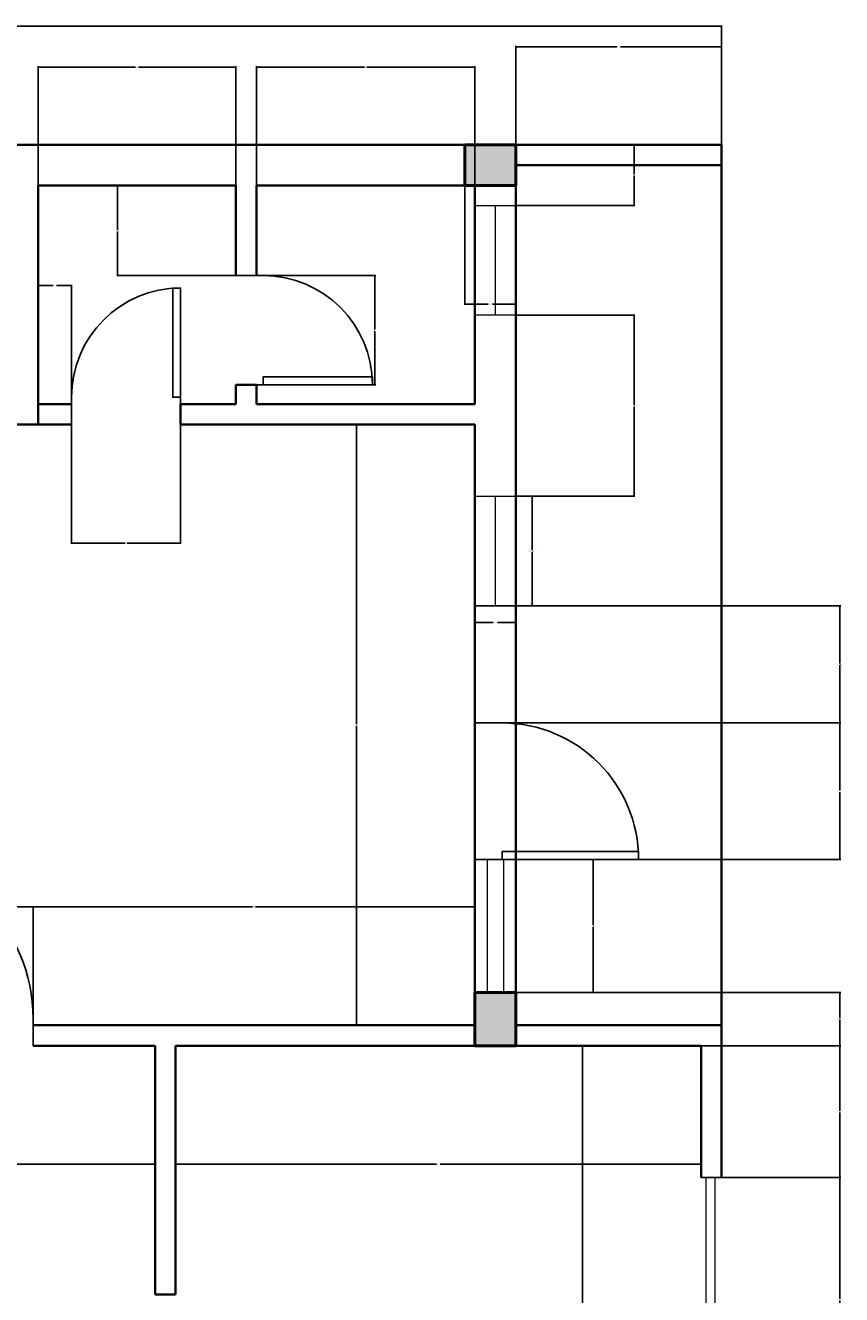
# Model space of a CAD drawing. Units: inches. Extents: x 229 to 651, y 108 to 681.
# Tile 4 of 4: x 472 to 651, y 402 to 681. Entities that reach past the tile are written whole.
import ezdxf

# ---------------------------------------------------------------- set-up
doc = ezdxf.new("R2010")
doc.units = ezdxf.units.IN
doc.header["$MEASUREMENT"] = 0
for name, color, linetype, lineweight in [('A-ANNO-DIMS', 2, 'Continuous', 18), ('A-COLS', 7, 'Continuous', 50), ('A-COLS-PATT', 5, 'Continuous', 13), ('A-DOOR', 3, 'Continuous', 25), ('A-GLAZ', 4, 'Continuous', 18), ('A-WALL', 7, 'Continuous', 35)]:
    doc.layers.add(name, color=color, linetype=linetype, lineweight=lineweight)
doc.styles.get("Standard").update_dxf_attribs({"font": 'arial.ttf'})
doc.dimstyles.get("Standard").update_dxf_attribs({"dimtxt": 0.18, "dimasz": 0.18, "dimexe": 0.18, "dimexo": 0.0625, "dimgap": 0.09, "dimtad": 0, "dimtih": 1, "dimtoh": 1, "dimdec": 4, "dimzin": 0, "dimdsep": 46, "dimtxsty": 'Standard', "dimcen": 0.09, "dimadec": 0, "dimazin": 0, "dimtfac": 1, "dimtdec": 4, "dimtofl": 0, "dimtmove": 0, "dimatfit": 3, "dimfxl": 1, "dimtolj": 1, "dimtzin": 0, "dimarcsym": 0})

# ---------------------------------------------------------------- blocks, each defined once
blk = doc.blocks.new('*U4')
for p, q in [((0, 0), (0, -6)), ((36, 0), (36, -6))]:
    blk.add_line(p, q)
blk.add_lwpolyline([(0, 0), (0, 36), (1.75, 36), (1.75, 0)], close=True)
blk.add_arc((0, 0), 36, 0, 90)
blk = doc.blocks.new('*U5')
for p, q in [((-24, 0), (-24, -6)), ((0, 0), (0, -6))]:
    blk.add_line(p, q)
blk.add_lwpolyline([(0, 0), (0, 24), (-1.75, 24), (-1.75, 0)], close=True)
blk.add_arc((0, 0), 24, 90, 180)
blk = doc.blocks.new('*U6')
for p, q in [((-30, 0), (-30, -6)), ((0, 0), (0, -6))]:
    blk.add_line(p, q)
blk.add_lwpolyline([(0, 0), (0, 30), (-1.75, 30), (-1.75, 0)], close=True)
blk.add_arc((0, 0), 30, 90, 180)
blk = doc.blocks.new('WIN-24IN-SINGLE')
for p, q in [((0, 24.08), (9, 24.08)), ((0, 0), (0, 24.08)), ((0, 24.08), (4.5, 24.08)), ((4.5, 24.08), (4.5, 0)), ((9, 24.08), (9, 0)), ((9, 0), (0, 0))]:
    blk.add_line(p, q)
blk = doc.blocks.new('*D11')
at = {"layer": 'A-ANNO-DIMS', "color": 0, "lineweight": -2, "transparency": 16777216}
for p, q in [((579.81, 577.83), (583.54, 577.83)), ((583.36, 577.65), (583.36, 565.97)), ((583.36, 553.93), (583.36, 565.6)), ((579.81, 553.75), (583.54, 553.75))]:
    blk.add_line(p, q, dxfattribs=at)
at = {"layer": 'A-ANNO-DIMS', "color": 0, "transparency": 16777216}
for points in [[(583.33, 577.65), (583.39, 577.65), (583.36, 577.83)], [(583.33, 553.93), (583.39, 553.93), (583.36, 553.75)]]:
    blk.add_solid(points, dxfattribs=at)
at = {"layer": 'Defpoints', "color": 0, "transparency": 16777216}
for p in [(579.74, 577.83), (583.36, 577.83), (579.74, 553.75)]:
    blk.add_point(p, dxfattribs=at)
at = {"layer": 'A-ANNO-DIMS', "color": 0, "transparency": 16777216, "insert": (583.36, 565.79), "char_height": 0.18, "attachment_point": 5}
blk.add_mtext('\\A1;WINDOW 24 TYP.', dxfattribs=at)
blk = doc.blocks.new('*D12')
at = {"layer": 'A-ANNO-DIMS', "color": 0, "lineweight": -2, "transparency": 16777216}
for p, q in [((570.74, 553.68), (570.74, 549.95)), ((579.74, 553.68), (579.74, 549.95)), ((570.92, 550.13), (574.79, 550.13)), ((579.56, 550.13), (575.7, 550.13))]:
    blk.add_line(p, q, dxfattribs=at)
at = {"layer": 'A-ANNO-DIMS', "color": 0, "transparency": 16777216}
for points in [[(570.92, 550.16), (570.92, 550.1), (570.74, 550.13)], [(579.56, 550.16), (579.56, 550.1), (579.74, 550.13)]]:
    blk.add_solid(points, dxfattribs=at)
at = {"layer": 'Defpoints', "color": 0, "transparency": 16777216}
for p in [(570.74, 553.75), (579.74, 553.75), (579.74, 550.13)]:
    blk.add_point(p, dxfattribs=at)
at = {"layer": 'A-ANNO-DIMS', "color": 0, "transparency": 16777216, "insert": (575.24, 550.13), "char_height": 0.18, "attachment_point": 5}
blk.add_mtext('\\A1;9 TYP.', dxfattribs=at)
blk = doc.blocks.new('*D13')
at = {"layer": 'A-ANNO-DIMS', "color": 0, "lineweight": -2, "transparency": 16777216}
for p, q in [((255.74, 655.15), (255.74, 681.3)), ((255.92, 681.12), (439.96, 681.12)), ((624.79, 681.12), (440.75, 681.12)), ((624.97, 655.15), (624.97, 681.3))]:
    blk.add_line(p, q, dxfattribs=at)
at = {"layer": 'A-ANNO-DIMS', "color": 0, "transparency": 16777216}
for points in [[(255.92, 681.15), (255.92, 681.09), (255.74, 681.12)], [(624.79, 681.15), (624.79, 681.09), (624.97, 681.12)]]:
    blk.add_solid(points, dxfattribs=at)
at = {"layer": 'Defpoints', "color": 0, "transparency": 16777216}
for p in [(624.97, 681.12), (255.74, 655.09), (624.97, 655.09)]:
    blk.add_point(p, dxfattribs=at)
at = {"layer": 'A-ANNO-DIMS', "color": 0, "transparency": 16777216, "insert": (440.36, 681.12), "char_height": 0.18, "attachment_point": 5}
blk.add_mtext('\\A1;369.2', dxfattribs=at)
blk = doc.blocks.new('*D15')
at = {"layer": 'A-ANNO-DIMS', "color": 0, "lineweight": -2, "transparency": 16777216}
for p, q in [((579.74, 650.65), (579.74, 676.8)), ((579.92, 676.62), (601.96, 676.62)), ((624.79, 676.62), (602.75, 676.62)), ((624.97, 650.65), (624.97, 676.8))]:
    blk.add_line(p, q, dxfattribs=at)
at = {"layer": 'A-ANNO-DIMS', "color": 0, "transparency": 16777216}
for points in [[(579.92, 676.65), (579.92, 676.59), (579.74, 676.62)], [(624.79, 676.65), (624.79, 676.59), (624.97, 676.62)]]:
    blk.add_solid(points, dxfattribs=at)
at = {"layer": 'Defpoints', "color": 0, "transparency": 16777216}
for p in [(624.97, 676.62), (579.74, 650.59), (624.97, 650.59)]:
    blk.add_point(p, dxfattribs=at)
at = {"layer": 'A-ANNO-DIMS', "color": 0, "transparency": 16777216, "insert": (602.36, 676.62), "char_height": 0.18, "attachment_point": 5}
blk.add_mtext('\\A1;45.23', dxfattribs=at)
blk = doc.blocks.new('*D17')
at = {"layer": 'A-ANNO-DIMS', "color": 0, "lineweight": -2, "transparency": 16777216}
for p, q in [((620.41, 457.09), (594.26, 457.09)), ((594.44, 456.91), (594.44, 397.27)), ((594.44, 337.27), (594.44, 396.9)), ((620.41, 337.09), (594.26, 337.09))]:
    blk.add_line(p, q, dxfattribs=at)
at = {"layer": 'A-ANNO-DIMS', "color": 0, "transparency": 16777216}
for points in [[(594.41, 456.91), (594.47, 456.91), (594.44, 457.09)], [(594.41, 337.27), (594.47, 337.27), (594.44, 337.09)]]:
    blk.add_solid(points, dxfattribs=at)
at = {"layer": 'Defpoints', "color": 0, "transparency": 16777216}
for p in [(594.44, 457.09), (620.47, 457.09), (620.47, 337.09)]:
    blk.add_point(p, dxfattribs=at)
at = {"layer": 'A-ANNO-DIMS', "color": 0, "transparency": 16777216, "insert": (594.44, 397.09), "char_height": 0.18, "attachment_point": 5}
blk.add_mtext('\\A1;120', dxfattribs=at)
blk = doc.blocks.new('*D22')
at = {"layer": 'A-ANNO-DIMS', "color": 0, "lineweight": -2, "transparency": 16777216}
for p, q in [((474.74, 646.15), (474.74, 672.3)), ((474.92, 672.12), (496.17, 672.12)), ((518.06, 672.12), (496.82, 672.12)), ((518.24, 646.15), (518.24, 672.3))]:
    blk.add_line(p, q, dxfattribs=at)
at = {"layer": 'A-ANNO-DIMS', "color": 0, "transparency": 16777216}
for points in [[(474.92, 672.15), (474.92, 672.09), (474.74, 672.12)], [(518.06, 672.15), (518.06, 672.09), (518.24, 672.12)]]:
    blk.add_solid(points, dxfattribs=at)
at = {"layer": 'Defpoints', "color": 0, "transparency": 16777216}
for p in [(518.24, 672.12), (474.74, 646.09), (518.24, 646.09)]:
    blk.add_point(p, dxfattribs=at)
at = {"layer": 'A-ANNO-DIMS', "color": 0, "transparency": 16777216, "insert": (496.49, 672.12), "char_height": 0.18, "attachment_point": 5}
blk.add_mtext('\\A1;43.5', dxfattribs=at)
blk = doc.blocks.new('*D23')
at = {"layer": 'A-ANNO-DIMS', "color": 0, "lineweight": -2, "transparency": 16777216}
for p, q in [((522.74, 646.15), (522.74, 672.3)), ((522.92, 672.12), (546.52, 672.12)), ((570.56, 672.12), (546.97, 672.12)), ((570.74, 646.15), (570.74, 672.3))]:
    blk.add_line(p, q, dxfattribs=at)
at = {"layer": 'A-ANNO-DIMS', "color": 0, "transparency": 16777216}
for points in [[(522.92, 672.15), (522.92, 672.09), (522.74, 672.12)], [(570.56, 672.15), (570.56, 672.09), (570.74, 672.12)]]:
    blk.add_solid(points, dxfattribs=at)
at = {"layer": 'Defpoints', "color": 0, "transparency": 16777216}
for p in [(570.74, 672.12), (522.74, 646.09), (570.74, 646.09)]:
    blk.add_point(p, dxfattribs=at)
at = {"layer": 'A-ANNO-DIMS', "color": 0, "transparency": 16777216, "insert": (546.74, 672.12), "char_height": 0.18, "attachment_point": 5}
blk.add_mtext('\\A1;48', dxfattribs=at)
blk = doc.blocks.new('*D25')
at = {"layer": 'A-ANNO-DIMS', "color": 0, "lineweight": -2, "transparency": 16777216}
for p, q in [((579.81, 655.09), (605.95, 655.09)), ((605.77, 654.91), (605.77, 648.58)), ((605.77, 641.9), (605.77, 648.22)), ((579.81, 641.72), (605.95, 641.72))]:
    blk.add_line(p, q, dxfattribs=at)
at = {"layer": 'A-ANNO-DIMS', "color": 0, "transparency": 16777216}
for points in [[(605.74, 654.91), (605.8, 654.91), (605.77, 655.09)], [(605.74, 641.9), (605.8, 641.9), (605.77, 641.72)]]:
    blk.add_solid(points, dxfattribs=at)
at = {"layer": 'Defpoints', "color": 0, "transparency": 16777216}
for p in [(579.74, 655.09), (579.74, 641.72), (605.77, 641.72)]:
    blk.add_point(p, dxfattribs=at)
at = {"layer": 'A-ANNO-DIMS', "color": 0, "transparency": 16777216, "insert": (605.77, 648.4), "char_height": 0.18, "attachment_point": 5}
blk.add_mtext('\\A1;13.37', dxfattribs=at)
blk = doc.blocks.new('*D26')
at = {"layer": 'A-ANNO-DIMS', "color": 0, "lineweight": -2, "transparency": 16777216}
for p, q in [((579.81, 617.63), (605.95, 617.63)), ((605.77, 617.45), (605.77, 597.91)), ((605.77, 578.01), (605.77, 597.55)), ((579.81, 577.83), (605.95, 577.83))]:
    blk.add_line(p, q, dxfattribs=at)
at = {"layer": 'A-ANNO-DIMS', "color": 0, "transparency": 16777216}
for points in [[(605.74, 617.45), (605.8, 617.45), (605.77, 617.63)], [(605.74, 578.01), (605.8, 578.01), (605.77, 577.83)]]:
    blk.add_solid(points, dxfattribs=at)
at = {"layer": 'Defpoints', "color": 0, "transparency": 16777216}
for p in [(579.74, 617.63), (579.74, 577.83), (605.77, 577.83)]:
    blk.add_point(p, dxfattribs=at)
at = {"layer": 'A-ANNO-DIMS', "color": 0, "transparency": 16777216, "insert": (605.77, 597.73), "char_height": 0.18, "attachment_point": 5}
blk.add_mtext('\\A1;39.804', dxfattribs=at)
blk = doc.blocks.new('*D27')
at = {"layer": 'A-ANNO-DIMS', "color": 0, "lineweight": -2, "transparency": 16777216}
for p, q in [((570.81, 553.75), (651.18, 553.75)), ((651, 553.57), (651, 541.07)), ((651, 528.2), (651, 540.7)), ((570.81, 528.02), (651.18, 528.02))]:
    blk.add_line(p, q, dxfattribs=at)
at = {"layer": 'A-ANNO-DIMS', "color": 0, "transparency": 16777216}
for points in [[(650.97, 553.57), (651.03, 553.57), (651, 553.75)], [(650.97, 528.2), (651.03, 528.2), (651, 528.02)]]:
    blk.add_solid(points, dxfattribs=at)
at = {"layer": 'Defpoints', "color": 0, "transparency": 16777216}
for p in [(570.74, 553.75), (570.74, 528.02), (651, 528.02)]:
    blk.add_point(p, dxfattribs=at)
at = {"layer": 'A-ANNO-DIMS', "color": 0, "transparency": 16777216, "insert": (651, 540.88), "char_height": 0.18, "attachment_point": 5}
blk.add_mtext('\\A1;25.725', dxfattribs=at)
blk = doc.blocks.new('*D28')
at = {"layer": 'A-ANNO-DIMS', "color": 0, "lineweight": -2, "transparency": 16777216}
for p, q in [((570.81, 528.02), (651.18, 528.02)), ((651, 527.84), (651, 513.2)), ((651, 498.2), (651, 512.84)), ((570.81, 498.02), (651.18, 498.02))]:
    blk.add_line(p, q, dxfattribs=at)
at = {"layer": 'A-ANNO-DIMS', "color": 0, "transparency": 16777216}
for points in [[(650.97, 527.84), (651.03, 527.84), (651, 528.02)], [(650.97, 498.2), (651.03, 498.2), (651, 498.02)]]:
    blk.add_solid(points, dxfattribs=at)
at = {"layer": 'Defpoints', "color": 0, "transparency": 16777216}
for p in [(570.74, 528.02), (651, 528.02), (570.74, 498.02)]:
    blk.add_point(p, dxfattribs=at)
at = {"layer": 'A-ANNO-DIMS', "color": 0, "transparency": 16777216, "insert": (651, 513.02), "char_height": 0.18, "attachment_point": 5}
blk.add_mtext('\\A1;30', dxfattribs=at)
blk = doc.blocks.new('*D29')
at = {"layer": 'A-ANNO-DIMS', "color": 0, "lineweight": -2, "transparency": 16777216}
for p, q in [((570.81, 498.02), (596.95, 498.02)), ((596.77, 497.84), (596.77, 483.6)), ((596.77, 469), (596.77, 483.24)), ((570.81, 468.82), (596.95, 468.82))]:
    blk.add_line(p, q, dxfattribs=at)
at = {"layer": 'A-ANNO-DIMS', "color": 0, "transparency": 16777216}
for points in [[(596.74, 497.84), (596.8, 497.84), (596.77, 498.02)], [(596.74, 469), (596.8, 469), (596.77, 468.82)]]:
    blk.add_solid(points, dxfattribs=at)
at = {"layer": 'Defpoints', "color": 0, "transparency": 16777216}
for p in [(570.74, 498.02), (570.74, 468.82), (596.77, 468.82)]:
    blk.add_point(p, dxfattribs=at)
at = {"layer": 'A-ANNO-DIMS', "color": 0, "transparency": 16777216, "insert": (596.77, 483.42), "char_height": 0.18, "attachment_point": 5}
blk.add_mtext('\\A1;29.205', dxfattribs=at)
blk = doc.blocks.new('*D32')
at = {"layer": 'A-ANNO-DIMS', "color": 0, "lineweight": -2, "transparency": 16777216}
for p, q in [((437.65, 461.65), (437.65, 487.8)), ((437.83, 487.62), (455.43, 487.62)), ((473.47, 487.62), (455.87, 487.62)), ((473.65, 461.65), (473.65, 487.8))]:
    blk.add_line(p, q, dxfattribs=at)
at = {"layer": 'A-ANNO-DIMS', "color": 0, "transparency": 16777216}
for points in [[(437.83, 487.65), (437.83, 487.59), (437.65, 487.62)], [(473.47, 487.65), (473.47, 487.59), (473.65, 487.62)]]:
    blk.add_solid(points, dxfattribs=at)
at = {"layer": 'Defpoints', "color": 0, "transparency": 16777216}
for p in [(473.65, 487.62), (437.65, 461.59), (473.65, 461.59)]:
    blk.add_point(p, dxfattribs=at)
at = {"layer": 'A-ANNO-DIMS', "color": 0, "transparency": 16777216, "insert": (455.65, 487.62), "char_height": 0.18, "attachment_point": 5}
blk.add_mtext('\\A1;36', dxfattribs=at)
blk = doc.blocks.new('*D33')
at = {"layer": 'A-ANNO-DIMS', "color": 0, "lineweight": -2, "transparency": 16777216}
for p, q in [((473.65, 461.65), (473.65, 487.8)), ((473.83, 487.62), (521.89, 487.62)), ((570.56, 487.62), (522.5, 487.62)), ((570.74, 461.65), (570.74, 487.8))]:
    blk.add_line(p, q, dxfattribs=at)
at = {"layer": 'A-ANNO-DIMS', "color": 0, "transparency": 16777216}
for points in [[(473.83, 487.65), (473.83, 487.59), (473.65, 487.62)], [(570.56, 487.65), (570.56, 487.59), (570.74, 487.62)]]:
    blk.add_solid(points, dxfattribs=at)
at = {"layer": 'Defpoints', "color": 0, "transparency": 16777216}
for p in [(570.74, 487.62), (473.65, 461.59), (570.74, 461.59)]:
    blk.add_point(p, dxfattribs=at)
at = {"layer": 'A-ANNO-DIMS', "color": 0, "transparency": 16777216, "insert": (522.2, 487.62), "char_height": 0.18, "attachment_point": 5}
blk.add_mtext('\\A1;97.1', dxfattribs=at)
blk = doc.blocks.new('*D34')
at = {"layer": 'A-ANNO-DIMS', "color": 0, "lineweight": -2, "transparency": 16777216}
for p, q in [((482.08, 593.52), (482.08, 567.38)), ((506.08, 593.52), (506.08, 567.38)), ((482.26, 567.56), (493.86, 567.56)), ((505.9, 567.56), (494.3, 567.56))]:
    blk.add_line(p, q, dxfattribs=at)
at = {"layer": 'A-ANNO-DIMS', "color": 0, "transparency": 16777216}
for points in [[(482.26, 567.59), (482.26, 567.53), (482.08, 567.56)], [(505.9, 567.59), (505.9, 567.53), (506.08, 567.56)]]:
    blk.add_solid(points, dxfattribs=at)
at = {"layer": 'Defpoints', "color": 0, "transparency": 16777216}
for p in [(482.08, 593.59), (506.08, 593.59), (482.08, 567.56)]:
    blk.add_point(p, dxfattribs=at)
at = {"layer": 'A-ANNO-DIMS', "color": 0, "transparency": 16777216, "insert": (494.08, 567.56), "char_height": 0.18, "attachment_point": 5}
blk.add_mtext('\\A1;24', dxfattribs=at)
blk = doc.blocks.new('*D35')
at = {"layer": 'A-ANNO-DIMS', "color": 0, "lineweight": -2, "transparency": 16777216}
for p, q in [((474.74, 598.15), (474.74, 624.3)), ((474.92, 624.12), (478.02, 624.12)), ((481.9, 624.12), (478.8, 624.12)), ((482.08, 598.15), (482.08, 624.3))]:
    blk.add_line(p, q, dxfattribs=at)
at = {"layer": 'A-ANNO-DIMS', "color": 0, "transparency": 16777216}
for points in [[(474.92, 624.15), (474.92, 624.09), (474.74, 624.12)], [(481.9, 624.15), (481.9, 624.09), (482.08, 624.12)]]:
    blk.add_solid(points, dxfattribs=at)
at = {"layer": 'Defpoints', "color": 0, "transparency": 16777216}
for p in [(482.08, 624.12), (474.74, 598.09), (482.08, 598.09)]:
    blk.add_point(p, dxfattribs=at)
at = {"layer": 'A-ANNO-DIMS', "color": 0, "transparency": 16777216, "insert": (478.41, 624.12), "char_height": 0.18, "attachment_point": 5}
blk.add_mtext('\\A1;7.333', dxfattribs=at)
blk = doc.blocks.new('*D36')
at = {"layer": 'A-ANNO-DIMS', "color": 0, "lineweight": -2, "transparency": 16777216}
for p, q in [((522.81, 626.33), (548.95, 626.33)), ((548.77, 626.15), (548.77, 614.51)), ((548.77, 602.51), (548.77, 614.14)), ((522.81, 602.33), (548.95, 602.33))]:
    blk.add_line(p, q, dxfattribs=at)
at = {"layer": 'A-ANNO-DIMS', "color": 0, "transparency": 16777216}
for points in [[(548.74, 626.15), (548.8, 626.15), (548.77, 626.33)], [(548.74, 602.51), (548.8, 602.51), (548.77, 602.33)]]:
    blk.add_solid(points, dxfattribs=at)
at = {"layer": 'Defpoints', "color": 0, "transparency": 16777216}
for p in [(522.74, 626.33), (522.74, 602.33), (548.77, 602.33)]:
    blk.add_point(p, dxfattribs=at)
at = {"layer": 'A-ANNO-DIMS', "color": 0, "transparency": 16777216, "insert": (548.77, 614.33), "char_height": 0.18, "attachment_point": 5}
blk.add_mtext('\\A1;24', dxfattribs=at)
blk = doc.blocks.new('*D37')
at = {"layer": 'A-ANNO-DIMS', "color": 0, "lineweight": -2, "transparency": 16777216}
for p, q in [((518.18, 646.09), (492.03, 646.09)), ((492.21, 645.91), (492.21, 636.39)), ((492.21, 626.51), (492.21, 636.02)), ((518.18, 626.33), (492.03, 626.33))]:
    blk.add_line(p, q, dxfattribs=at)
at = {"layer": 'A-ANNO-DIMS', "color": 0, "transparency": 16777216}
for points in [[(492.18, 645.91), (492.24, 645.91), (492.21, 646.09)], [(492.18, 626.51), (492.24, 626.51), (492.21, 626.33)]]:
    blk.add_solid(points, dxfattribs=at)
at = {"layer": 'Defpoints', "color": 0, "transparency": 16777216}
for p in [(492.21, 646.09), (518.24, 646.09), (518.24, 626.33)]:
    blk.add_point(p, dxfattribs=at)
at = {"layer": 'A-ANNO-DIMS', "color": 0, "transparency": 16777216, "insert": (492.21, 636.21), "char_height": 0.18, "attachment_point": 5}
blk.add_mtext('\\A1;19.76', dxfattribs=at)
blk = doc.blocks.new('*D41')
at = {"layer": 'A-ANNO-DIMS', "color": 0, "lineweight": -2, "transparency": 16777216}
for p, q in [((311.65, 457.02), (311.65, 430.88)), ((500.47, 457.02), (500.47, 430.88)), ((311.83, 431.06), (405.61, 431.06)), ((500.29, 431.06), (406.51, 431.06))]:
    blk.add_line(p, q, dxfattribs=at)
at = {"layer": 'A-ANNO-DIMS', "color": 0, "transparency": 16777216}
for points in [[(311.83, 431.09), (311.83, 431.03), (311.65, 431.06)], [(500.29, 431.09), (500.29, 431.03), (500.47, 431.06)]]:
    blk.add_solid(points, dxfattribs=at)
at = {"layer": 'Defpoints', "color": 0, "transparency": 16777216}
for p in [(311.65, 457.09), (500.47, 457.09), (311.65, 431.06)]:
    blk.add_point(p, dxfattribs=at)
at = {"layer": 'A-ANNO-DIMS', "color": 0, "transparency": 16777216, "insert": (406.06, 431.06), "char_height": 0.18, "attachment_point": 5}
blk.add_mtext('\\A1;188.82', dxfattribs=at)
blk = doc.blocks.new('*D42')
at = {"layer": 'A-ANNO-DIMS', "color": 0, "lineweight": -2, "transparency": 16777216}
for p, q in [((504.97, 457.02), (504.97, 430.88)), ((620.47, 457.02), (620.47, 430.88)), ((505.15, 431.06), (562.33, 431.06)), ((620.29, 431.06), (563.11, 431.06))]:
    blk.add_line(p, q, dxfattribs=at)
at = {"layer": 'A-ANNO-DIMS', "color": 0, "transparency": 16777216}
for points in [[(505.15, 431.09), (505.15, 431.03), (504.97, 431.06)], [(620.29, 431.09), (620.29, 431.03), (620.47, 431.06)]]:
    blk.add_solid(points, dxfattribs=at)
at = {"layer": 'Defpoints', "color": 0, "transparency": 16777216}
for p in [(504.97, 457.09), (620.47, 457.09), (504.97, 431.06)]:
    blk.add_point(p, dxfattribs=at)
at = {"layer": 'A-ANNO-DIMS', "color": 0, "transparency": 16777216, "insert": (562.72, 431.06), "char_height": 0.18, "attachment_point": 5}
blk.add_mtext('\\A1;115.5', dxfattribs=at)
blk = doc.blocks.new('*D45')
at = {"layer": 'A-ANNO-DIMS', "color": 0, "lineweight": -2, "transparency": 16777216}
for p, q in [((620.53, 428.12), (651.18, 428.12)), ((651, 427.94), (651, 401.49)), ((651, 374.68), (651, 401.13)), ((620.53, 374.5), (651.18, 374.5))]:
    blk.add_line(p, q, dxfattribs=at)
at = {"layer": 'A-ANNO-DIMS', "color": 0, "transparency": 16777216}
for points in [[(650.97, 427.94), (651.03, 427.94), (651, 428.12)], [(650.97, 374.68), (651.03, 374.68), (651, 374.5)]]:
    blk.add_solid(points, dxfattribs=at)
at = {"layer": 'Defpoints', "color": 0, "transparency": 16777216}
for p in [(620.47, 428.12), (651, 428.12), (620.47, 374.5)]:
    blk.add_point(p, dxfattribs=at)
at = {"layer": 'A-ANNO-DIMS', "color": 0, "transparency": 16777216, "insert": (651, 401.31), "char_height": 0.18, "attachment_point": 5}
blk.add_mtext('\\A1;53.63', dxfattribs=at)
blk = doc.blocks.new('*D46')
at = {"layer": 'A-ANNO-DIMS', "color": 0, "lineweight": -2, "transparency": 16777216}
for p, q in [((620.53, 457.09), (651.18, 457.09)), ((651, 456.91), (651, 442.79)), ((651, 428.3), (651, 442.42)), ((620.53, 428.12), (651.18, 428.12))]:
    blk.add_line(p, q, dxfattribs=at)
at = {"layer": 'A-ANNO-DIMS', "color": 0, "transparency": 16777216}
for points in [[(650.97, 456.91), (651.03, 456.91), (651, 457.09)], [(650.97, 428.3), (651.03, 428.3), (651, 428.12)]]:
    blk.add_solid(points, dxfattribs=at)
at = {"layer": 'Defpoints', "color": 0, "transparency": 16777216}
for p in [(620.47, 457.09), (651, 457.09), (620.47, 428.12)]:
    blk.add_point(p, dxfattribs=at)
at = {"layer": 'A-ANNO-DIMS', "color": 0, "transparency": 16777216, "insert": (651, 442.61), "char_height": 0.18, "attachment_point": 5}
blk.add_mtext('\\A1;28.963', dxfattribs=at)
blk = doc.blocks.new('*D72')
at = {"layer": 'A-ANNO-DIMS', "color": 0, "lineweight": -2, "transparency": 16777216}
for p, q in [((570.68, 593.59), (544.53, 593.59)), ((544.71, 593.41), (544.71, 527.77)), ((544.71, 461.77), (544.71, 527.4)), ((570.68, 461.59), (544.53, 461.59))]:
    blk.add_line(p, q, dxfattribs=at)
at = {"layer": 'A-ANNO-DIMS', "color": 0, "transparency": 16777216}
for points in [[(544.68, 593.41), (544.74, 593.41), (544.71, 593.59)], [(544.68, 461.77), (544.74, 461.77), (544.71, 461.59)]]:
    blk.add_solid(points, dxfattribs=at)
at = {"layer": 'Defpoints', "color": 0, "transparency": 16777216}
for p in [(544.71, 593.59), (570.74, 593.59), (570.74, 461.59)]:
    blk.add_point(p, dxfattribs=at)
at = {"layer": 'A-ANNO-DIMS', "color": 0, "transparency": 16777216, "insert": (544.71, 527.59), "char_height": 0.18, "attachment_point": 5}
blk.add_mtext('\\A1;132', dxfattribs=at)
blk = doc.blocks.new('*D74')
at = {"layer": 'A-ANNO-DIMS', "color": 0, "lineweight": -2, "transparency": 16777216}
for p, q in [((568.54, 646.02), (568.54, 619.88)), ((579.74, 646.02), (579.74, 619.88)), ((568.72, 620.06), (573.69, 620.06)), ((579.56, 620.06), (574.6, 620.06))]:
    blk.add_line(p, q, dxfattribs=at)
at = {"layer": 'A-ANNO-DIMS', "color": 0, "transparency": 16777216}
for points in [[(568.72, 620.09), (568.72, 620.03), (568.54, 620.06)], [(579.56, 620.09), (579.56, 620.03), (579.74, 620.06)]]:
    blk.add_solid(points, dxfattribs=at)
at = {"layer": 'Defpoints', "color": 0, "transparency": 16777216}
for p in [(568.54, 646.09), (579.74, 646.09), (568.54, 620.06)]:
    blk.add_point(p, dxfattribs=at)
at = {"layer": 'A-ANNO-DIMS', "color": 0, "transparency": 16777216, "insert": (574.14, 620.06), "char_height": 0.18, "attachment_point": 5}
blk.add_mtext('\\A1;11.207', dxfattribs=at)
blk = doc.blocks.new('*D78')
at = {"layer": 'A-ANNO-DIMS', "color": 0, "lineweight": -2, "transparency": 16777216}
for p, q in [((579.81, 468.82), (651.18, 468.82)), ((651, 468.64), (651, 463.13)), ((651, 457.27), (651, 462.77)), ((579.81, 457.09), (651.18, 457.09))]:
    blk.add_line(p, q, dxfattribs=at)
at = {"layer": 'A-ANNO-DIMS', "color": 0, "transparency": 16777216}
for points in [[(650.97, 468.64), (651.03, 468.64), (651, 468.82)], [(650.97, 457.27), (651.03, 457.27), (651, 457.09)]]:
    blk.add_solid(points, dxfattribs=at)
at = {"layer": 'Defpoints', "color": 0, "transparency": 16777216}
for p in [(579.74, 468.82), (579.74, 457.09), (651, 457.09)]:
    blk.add_point(p, dxfattribs=at)
at = {"layer": 'A-ANNO-DIMS', "color": 0, "transparency": 16777216, "insert": (651, 462.95), "char_height": 0.18, "attachment_point": 5}
blk.add_mtext('\\A1;11.73', dxfattribs=at)

msp = doc.modelspace()

# ---------------------------------------------------------------- hatches: boundary and pattern name
at = {"layer": 'A-COLS-PATT'}
h = msp.add_hatch(color=256, dxfattribs=at)
h.dxf.hatch_style = 1
h.paths.add_polyline_path([(264.7698, 655.0869), (255.744, 655.0869), (255.744, 646.0869), (264.7698, 646.0869)])
h.paths.add_polyline_path([(428.5355, 655.0869), (414.8518, 655.0869), (414.8518, 646.0869), (428.5355, 646.0869)])
h.paths.add_polyline_path([(579.744, 655.0869), (568.5366, 655.0869), (568.5366, 646.0869), (570.744, 646.0869), (579.744, 646.0869)])
h.paths.add_polyline_path([(579.744, 468.8158), (570.744, 468.8158), (570.744, 457.0869), (579.744, 457.0869)])
h.paths.add_polyline_path([(422.244, 467.874), (416.0718, 467.874), (416.0718, 457.0869), (422.244, 457.0869)])
h.paths.add_polyline_path([(264.744, 465.8018), (255.744, 465.8018), (255.744, 453.3882), (264.744, 453.3882), (264.744, 457.0869)])
h.paths.add_polyline_path([(264.744, 337.0869), (255.744, 337.0869), (255.744, 328.0161), (264.744, 328.0161)])
h.paths.add_polyline_path([(425.426, 337.0869), (411.84, 337.0869), (411.84, 328.0869), (425.426, 328.0869)])
h.paths.add_polyline_path([(579.744, 337.0869), (570.744, 337.0869), (570.744, 328.0869), (579.744, 328.0869)])
h.paths.add_polyline_path([(579.744, 188.4262), (570.744, 188.4262), (570.744, 178.0508), (579.744, 178.0508)])
h.paths.add_polyline_path([(413.7248, 169.0053), (405.843, 169.0053), (405.843, 162.8404), (413.7248, 162.8404)])
h.paths.add_polyline_path([(264.744, 180.6917), (255.744, 180.6917), (255.744, 171.3369), (264.744, 171.3369)])

# ---------------------------------------------------------------- linework, layer by layer
at = {"layer": 'A-COLS'}
for p, q in [((579.744, 655.0869), (568.5366, 655.0869)), ((568.5366, 655.0869), (568.5366, 646.0869)), ((579.744, 646.0869), (579.744, 655.0869)), ((568.5366, 646.0869), (570.744, 646.0869)), ((570.744, 646.0869), (579.744, 646.0869)), ((570.744, 468.8158), (579.744, 468.8158)), ((570.744, 457.0869), (570.744, 468.8158)), ((579.744, 468.8158), (579.744, 457.0869)), ((579.744, 457.0869), (570.744, 457.0869))]:
    msp.add_line(p, q, dxfattribs=at)
at = {"layer": 'A-GLAZ'}
for p, q in [((570.744, 498.021), (570.744, 468.8158)), ((579.744, 498.021), (570.744, 498.021)), ((573.4744, 498.021), (573.4744, 468.8158)), ((577.1433, 468.8158), (577.1433, 498.021)), ((579.744, 468.8158), (579.744, 498.021)), ((570.744, 468.8158), (579.744, 468.8158)), ((573.4744, 468.8158), (577.1433, 468.8158)), ((624.9705, 428.1237), (620.4705, 428.1237)), ((621.6316, 374.4959), (621.6316, 428.1237)), ((621.6316, 428.1237), (623.4874, 428.1237)), ((623.4874, 428.1237), (623.4874, 374.4959))]:
    msp.add_line(p, q, dxfattribs=at)
at = {"layer": 'A-WALL'}
for p, q in [((255.744, 655.0869), (579.744, 655.0869)), ((579.744, 655.0869), (579.744, 461.5869)), ((579.744, 655.0869), (624.9705, 655.0869)), ((624.9705, 650.5869), (624.9705, 655.0869)), ((624.9705, 650.5869), (624.9705, 655.0869)), ((624.9705, 652.8369), (624.9705, 655.0869)), ((624.9705, 459.3369), (624.9705, 652.8369)), ((579.744, 650.5869), (624.9705, 650.5869)), ((474.744, 593.5869), (474.744, 646.0869)), ((474.744, 646.0869), (518.244, 646.0869)), ((518.244, 646.0869), (518.244, 626.3253)), ((522.744, 646.0869), (522.744, 626.3253)), ((522.744, 646.0869), (570.744, 646.0869)), ((570.744, 646.0869), (570.744, 598.0869)), ((522.744, 602.3253), (518.244, 602.3253)), ((518.244, 602.3253), (518.244, 598.0869)), ((522.744, 602.3253), (522.744, 598.0869)), ((482.0771, 598.0869), (474.744, 598.0869)), ((518.244, 598.0869), (506.0771, 598.0869)), ((506.0771, 593.5869), (506.0771, 598.0869)), ((522.744, 598.0869), (570.744, 598.0869)), ((422.244, 593.5869), (474.744, 593.5869)), ((482.0771, 593.5869), (474.744, 593.5869)), ((518.244, 593.5869), (506.0771, 593.5869)), ((518.244, 593.5869), (570.744, 593.5869)), ((570.744, 593.5869), (570.744, 461.5869)), ((479.5364, 461.5869), (473.6462, 461.5869)), ((473.6462, 461.5869), (474.744, 461.5869)), ((474.744, 461.5869), (505.1177, 461.5869)), ((518.244, 461.5869), (501.1973, 461.5869)), ((518.244, 461.5869), (570.744, 461.5869)), ((570.744, 461.5869), (570.744, 457.0869)), ((624.9705, 461.5869), (579.744, 461.5869)), ((579.744, 461.5869), (579.744, 457.0869)), ((624.9705, 457.0869), (624.9705, 461.5869)), ((473.6462, 457.0869), (475.1505, 457.0869)), ((473.6462, 457.0869), (475.1505, 457.0869)), ((475.1505, 457.0869), (481.0885, 457.0869)), ((479.6505, 457.0869), (500.4705, 457.0869)), ((500.4705, 457.0869), (500.4705, 402.4166)), ((504.9705, 457.0869), (504.9705, 402.4166)), ((504.9705, 457.0869), (586.846, 457.0869)), ((570.744, 457.0869), (594.744, 457.0869)), ((570.744, 457.0869), (575.244, 457.0869)), ((594.744, 457.0869), (599.6505, 457.0869)), ((599.6505, 457.0869), (620.4705, 457.0869)), ((604.1505, 457.0869), (618.744, 457.0869)), ((620.4705, 457.0869), (620.4705, 428.1237)), ((624.9705, 457.0869), (624.9705, 428.1237)), ((504.9705, 402.4166), (500.4705, 402.4166))]:
    msp.add_line(p, q, dxfattribs=at)

# ---------------------------------------------------------------- block references
at = {"layer": 'A-DOOR', "rotation": 270}
for name, p in [('*U5', (524.244, 602.3253)), ('*U6', (576.744, 498.021))]:
    msp.add_blockref(name, p, dxfattribs=at)
at = {"layer": 'A-DOOR'}
for name, p in [('*U5', (506.0771, 599.5869)), ('*U4', (437.6462, 463.0869))]:
    msp.add_blockref(name, p, dxfattribs=at)
at = {"layer": 'A-GLAZ'}
for p in [(570.744, 617.634), (570.744, 553.7463)]:
    msp.add_blockref('WIN-24IN-SINGLE', p, dxfattribs=at)

# ---------------------------------------------------------------- dimensions: what is measured, and where the dimension line sits
at = {"layer": 'A-ANNO-DIMS'}
for base, p1, p2, override, picture, middle in [((624.9705, 681.1169), (255.744, 655.0869), (624.9705, 655.0869), {"dimdec": 1, "dimlfac": 1, "dimrnd": 0, "dimzin": 0, "dimdsep": 46, "dimlunit": 2}, '*D13', (440.3573, 681.1169)), ((624.9705, 676.6169), (579.744, 650.5869), (624.9705, 650.5869), {"dimdec": 2, "dimlfac": 1, "dimrnd": 0, "dimzin": 0, "dimdsep": 46, "dimlunit": 2}, '*D15', (602.3573, 676.6169)), ((518.244, 672.1169), (474.744, 646.0869), (518.244, 646.0869), {"dimdec": 1, "dimlfac": 1, "dimrnd": 0, "dimzin": 0, "dimdsep": 46, "dimlunit": 2}, '*D22', (496.494, 672.1169)), ((570.744, 672.1169), (522.744, 646.0869), (570.744, 646.0869), {"dimdec": 0, "dimlfac": 1, "dimrnd": 0, "dimzin": 0, "dimdsep": 46, "dimlunit": 2}, '*D23', (546.744, 672.1169)), ((473.6462, 487.6169), (437.6462, 461.5869), (473.6462, 461.5869), {"dimdec": 0, "dimlfac": 1, "dimrnd": 0, "dimzin": 0, "dimdsep": 46, "dimlunit": 2}, '*D32', (455.6462, 487.6169)), ((570.744, 487.6169), (473.6462, 461.5869), (570.744, 461.5869), {"dimdec": 1, "dimlfac": 1, "dimrnd": 0, "dimzin": 0, "dimdsep": 46, "dimlunit": 2}, '*D33', (522.1951, 487.6169))]:
    dim = msp.add_linear_dim(base=base, p1=p1, p2=p2, dimstyle='Standard', override=override, dxfattribs=at)
    dim.commit()
    dim.dimension.update_dxf_attribs({"geometry": picture, "text_midpoint": middle})
for base, p1, p2, angle, override, picture, middle in [((605.774, 641.7175), (579.744, 655.0869), (579.744, 641.7175), 270, {"dimdec": 2, "dimlfac": 1, "dimrnd": 0, "dimzin": 0, "dimdsep": 46, "dimlunit": 2}, '*D25', (605.774, 648.4022)), ((492.214, 646.0869), (518.244, 626.3253), (518.244, 646.0869), 90, {"dimdec": 2, "dimlfac": 1, "dimrnd": 0, "dimzin": 0, "dimdsep": 46, "dimlunit": 2}, '*D37', (492.214, 636.2061)), ((568.5366, 620.0569), (579.744, 646.0869), (568.5366, 646.0869), 180, {"dimdec": 3, "dimlfac": 1, "dimrnd": 0, "dimzin": 0, "dimdsep": 46, "dimlunit": 2}, '*D74', (574.1403, 620.0569)), ((548.774, 602.3253), (522.744, 626.3253), (522.744, 602.3253), 270, {"dimdec": 0, "dimlfac": 1, "dimrnd": 0, "dimzin": 0, "dimdsep": 46, "dimlunit": 2}, '*D36', (548.774, 614.3253)), ((482.0771, 624.1169), (474.744, 598.0869), (482.0771, 598.0869), 0, {"dimdec": 3, "dimlfac": 1, "dimrnd": 0, "dimzin": 0, "dimdsep": 46, "dimlunit": 2}, '*D35', (478.4105, 624.1169)), ((605.774, 577.8297), (579.744, 617.6339), (579.744, 577.8297), 270, {"dimdec": 3, "dimlfac": 1, "dimrnd": 0, "dimzin": 0, "dimdsep": 46, "dimlunit": 2}, '*D26', (605.774, 597.7318)), ((482.0771, 567.5569), (506.0771, 593.5869), (482.0771, 593.5869), 180, {"dimdec": 0, "dimlfac": 1, "dimrnd": 0, "dimzin": 0, "dimdsep": 46, "dimlunit": 2}, '*D34', (494.0771, 567.5569)), ((544.714, 593.5869), (570.744, 461.5869), (570.744, 593.5869), 90, {"dimdec": 0, "dimlfac": 1, "dimrnd": 0, "dimzin": 0, "dimdsep": 46, "dimlunit": 2}, '*D72', (544.714, 527.5869)), ((651.0005, 528.021), (570.744, 553.7461), (570.744, 528.021), 90, {"dimdec": 3, "dimlfac": 1, "dimrnd": 0, "dimzin": 0, "dimdsep": 46, "dimlunit": 2}, '*D27', (651.0005, 540.8836)), ((651.0005, 528.021), (570.744, 498.021), (570.744, 528.021), 90, {"dimdec": 0, "dimlfac": 1, "dimrnd": 0, "dimzin": 0, "dimdsep": 46, "dimlunit": 2}, '*D28', (651.0005, 513.021)), ((596.774, 468.8158), (570.744, 498.021), (570.744, 468.8158), 270, {"dimdec": 3, "dimlfac": 1, "dimrnd": 0, "dimzin": 0, "dimdsep": 46, "dimlunit": 2}, '*D29', (596.774, 483.4184)), ((651.0005, 457.0869), (579.744, 468.8158), (579.744, 457.0869), 90, {"dimdec": 2, "dimlfac": 1, "dimrnd": 0, "dimzin": 0, "dimdsep": 46, "dimlunit": 2}, '*D78', (651.0005, 462.9513)), ((311.6505, 431.0569), (500.4705, 457.0869), (311.6505, 457.0869), 180, {"dimdec": 2, "dimlfac": 1, "dimrnd": 0, "dimzin": 0, "dimdsep": 46, "dimlunit": 2}, '*D41', (406.0605, 431.0569)), ((504.9705, 431.0569), (620.4705, 457.0869), (504.9705, 457.0869), 180, {"dimdec": 1, "dimlfac": 1, "dimrnd": 0, "dimzin": 0, "dimdsep": 46, "dimlunit": 2}, '*D42', (562.7205, 431.0569)), ((594.4405, 457.0869), (620.4705, 337.0869), (620.4705, 457.0869), 90, {"dimdec": 0, "dimlfac": 1, "dimrnd": 0, "dimzin": 0, "dimdsep": 46, "dimlunit": 2}, '*D17', (594.4405, 397.0869)), ((651.0005, 457.0869), (620.4705, 428.1237), (620.4705, 457.0869), 90, {"dimdec": 3, "dimlfac": 1, "dimrnd": 0, "dimzin": 0, "dimdsep": 46, "dimlunit": 2}, '*D46', (651.0005, 442.6053)), ((651.0005, 428.1237), (620.4705, 374.4959), (620.4705, 428.1237), 90, {"dimdec": 2, "dimlfac": 1, "dimrnd": 0, "dimzin": 0, "dimdsep": 46, "dimlunit": 2}, '*D45', (651.0005, 401.3098))]:
    dim = msp.add_linear_dim(base=base, p1=p1, p2=p2, angle=angle, dimstyle='Standard', override=override, dxfattribs=at)
    dim.commit()
    dim.dimension.update_dxf_attribs({"geometry": picture, "text_midpoint": middle})
dim = msp.add_linear_dim(base=(583.3566, 577.8297), p1=(579.744, 553.7461), p2=(579.744, 577.8297), angle=90, text='WINDOW <> TYP.', dimstyle='Standard', override={"dimdec": 0, "dimlfac": 1, "dimrnd": 0, "dimzin": 0, "dimdsep": 46, "dimlunit": 2}, dxfattribs=at)
dim.commit()
dim.dimension.update_dxf_attribs({"geometry": '*D11', "text_midpoint": (583.3566, 565.7879)})
dim = msp.add_linear_dim(base=(579.744, 550.1336), p1=(570.744, 553.7461), p2=(579.744, 553.7461), text='<> TYP.', dimstyle='Standard', override={"dimdec": 0, "dimlfac": 1, "dimrnd": 0, "dimzin": 0, "dimdsep": 46, "dimlunit": 2}, dxfattribs=at)
dim.commit()
dim.dimension.update_dxf_attribs({"geometry": '*D12', "text_midpoint": (575.244, 550.1336)})

doc.saveas('drawing.dxf')
